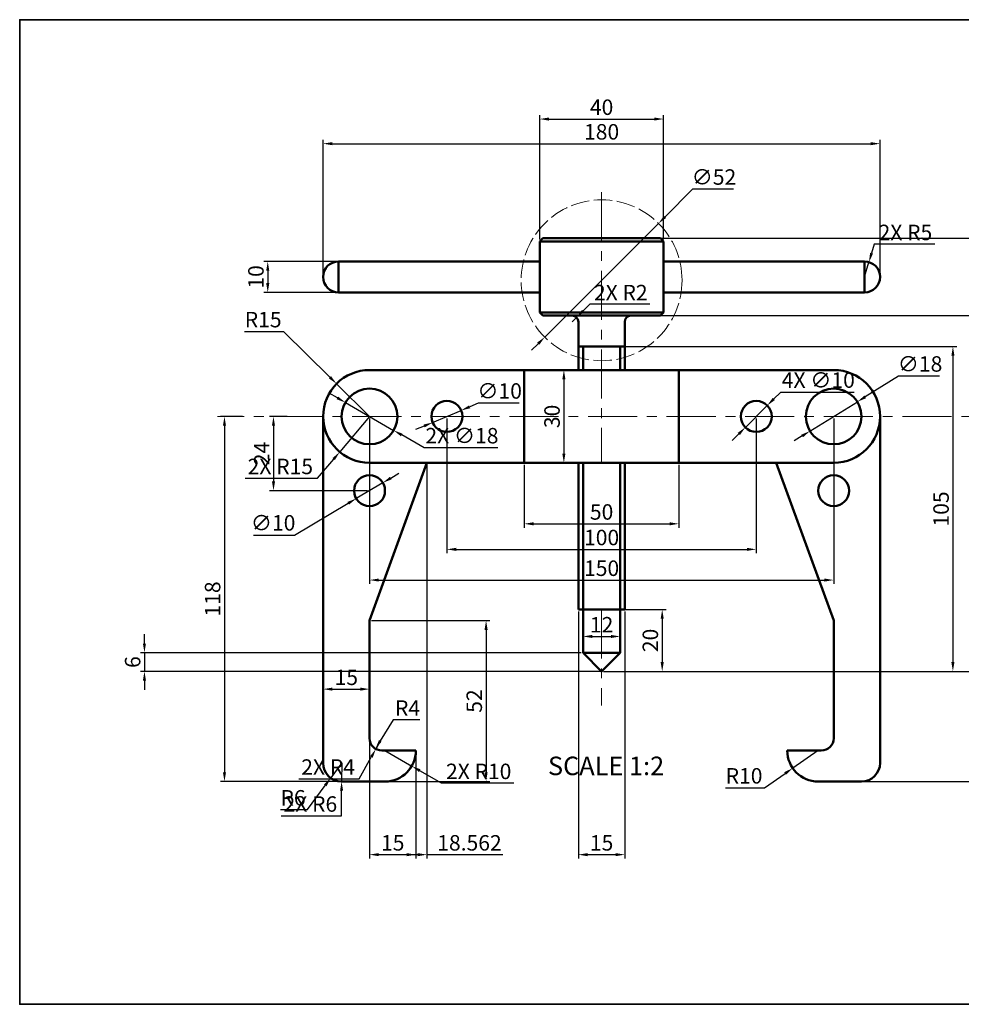
# Model space of a CAD drawing. Units: millimetres. Extents: x 535 to 1031, y 167 to 485.
# Tile 1 of 2: x 535 to 839, y 167 to 485. Entities that reach past the tile are written whole.
import ezdxf

# ---------------------------------------------------------------- set-up
doc = ezdxf.new("R2010")
doc.units = ezdxf.units.MM
doc.header["$LTSCALE"] = 0.5
doc.linetypes.add('ACAD_ISO02W100', pattern=[15, 12, -3])
doc.linetypes.add('CENTER', pattern=[50.8, 31.75, -6.35, 6.35, -6.35])
for name, color, linetype, lineweight in [('M-CNTR', 1, 'CENTER', 18), ('M-CONS', 8, 'ACAD_ISO02W100', 18), ('M-DIMS', 2, 'Continuous', 25), ('M-OUTL', 7, 'Continuous', 50), ('M-TEXT', 7, 'Continuous', 25), ('M-TTLB', 7, 'Continuous', 35)]:
    doc.layers.add(name, color=color, linetype=linetype, lineweight=lineweight)
doc.styles.get("Standard").update_dxf_attribs({"font": 'arial.ttf'})
doc.dimstyles.new('ISO-25', dxfattribs={"dimtxt": 5, "dimasz": 3, "dimexe": 1.25, "dimexo": 0.625, "dimtad": 1, "dimtoh": 1, "dimdec": 1, "dimtxsty": 'Standard', "dimcen": 2.5, "dimadec": 0, "dimazin": 0, "dimtfac": 1, "dimtdec": 1, "dimtmove": 0, "dimatfit": 3, "dimfxl": 1, "dimarcsym": 0})

# ---------------------------------------------------------------- blocks, each defined once
blk = doc.blocks.new('*D1')
at = {"layer": 'Defpoints', "color": 0, "transparency": 16777216}
for p in [(622.01, 356.84), (616.92, 332.84), (647.96, 332.84)]:
    blk.add_point(p, dxfattribs=at)
at = {"layer": 'M-DIMS', "color": 0, "lineweight": -2, "transparency": 16777216}
for p, q in [((621.39, 356.84), (615.67, 356.84)), ((616.92, 353.84), (616.92, 335.84)), ((647.33, 332.84), (615.67, 332.84))]:
    blk.add_line(p, q, dxfattribs=at)
at = {"layer": 'M-DIMS', "color": 0, "transparency": 16777216}
for points in [[(616.42, 353.84), (617.42, 353.84), (616.92, 356.84)], [(616.42, 335.84), (617.42, 335.84), (616.92, 332.84)]]:
    blk.add_solid(points, dxfattribs=at)
at = {"layer": 'M-DIMS', "color": 0, "transparency": 16777216, "insert": (613.78, 344.84), "char_height": 5, "attachment_point": 5, "rotation": 90}
blk.add_mtext('24', dxfattribs=at)
blk = doc.blocks.new('*D2')
at = {"layer": 'Defpoints', "color": 0, "transparency": 16777216}
for p in [(607.52, 356.84), (601.08, 238.84), (645.96, 238.84)]:
    blk.add_point(p, dxfattribs=at)
at = {"layer": 'M-DIMS', "color": 0, "lineweight": -2, "transparency": 16777216}
for p, q in [((606.9, 356.84), (599.83, 356.84)), ((601.08, 353.84), (601.08, 241.84)), ((645.33, 238.84), (599.83, 238.84))]:
    blk.add_line(p, q, dxfattribs=at)
at = {"layer": 'M-DIMS', "color": 0, "transparency": 16777216}
for points in [[(600.58, 353.84), (601.58, 353.84), (601.08, 356.84)], [(600.58, 241.84), (601.58, 241.84), (601.08, 238.84)]]:
    blk.add_solid(points, dxfattribs=at)
at = {"layer": 'M-DIMS', "color": 0, "transparency": 16777216, "insert": (597.9, 297.84), "char_height": 5, "attachment_point": 5, "rotation": 90}
blk.add_mtext('118', dxfattribs=at)
blk = doc.blocks.new('*D3')
at = {"layer": 'Defpoints', "color": 0, "transparency": 16777216}
for p in [(647.96, 290.84), (647.96, 238.84), (685.63, 238.84)]:
    blk.add_point(p, dxfattribs=at)
at = {"layer": 'M-DIMS', "color": 0, "lineweight": -2, "transparency": 16777216}
for p, q in [((648.58, 290.84), (686.88, 290.84)), ((685.63, 287.84), (685.63, 241.84)), ((648.58, 238.84), (686.88, 238.84))]:
    blk.add_line(p, q, dxfattribs=at)
at = {"layer": 'M-DIMS', "color": 0, "transparency": 16777216}
for points in [[(685.13, 287.84), (686.13, 287.84), (685.63, 290.84)], [(685.13, 241.84), (686.13, 241.84), (685.63, 238.84)]]:
    blk.add_solid(points, dxfattribs=at)
at = {"layer": 'M-DIMS', "color": 0, "transparency": 16777216, "insert": (682.45, 264.84), "char_height": 5, "attachment_point": 5, "rotation": 90}
blk.add_mtext('52', dxfattribs=at)
blk = doc.blocks.new('*D4')
at = {"layer": 'Defpoints', "color": 0, "transparency": 16777216}
for p in [(647.96, 268.69), (632.96, 265), (647.96, 265)]:
    blk.add_point(p, dxfattribs=at)
at = {"layer": 'M-DIMS', "color": 0, "lineweight": -2, "transparency": 16777216}
for p, q in [((632.96, 265.62), (632.96, 269.94)), ((635.96, 268.69), (644.96, 268.69)), ((647.96, 265.62), (647.96, 269.94))]:
    blk.add_line(p, q, dxfattribs=at)
at = {"layer": 'M-DIMS', "color": 0, "transparency": 16777216}
for points in [[(635.96, 269.19), (635.96, 268.19), (632.96, 268.69)], [(644.96, 269.19), (644.96, 268.19), (647.96, 268.69)]]:
    blk.add_solid(points, dxfattribs=at)
at = {"layer": 'M-DIMS', "color": 0, "transparency": 16777216, "insert": (640.46, 271.87), "char_height": 5, "attachment_point": 5}
blk.add_mtext('15', dxfattribs=at)
blk = doc.blocks.new('*D5')
at = {"layer": 'Defpoints', "color": 0, "transparency": 16777216}
for p in [(722.96, 294.43), (722.96, 274.43), (742.54, 274.43)]:
    blk.add_point(p, dxfattribs=at)
at = {"layer": 'M-DIMS', "color": 0, "lineweight": -2, "transparency": 16777216}
for p, q in [((723.58, 294.43), (743.79, 294.43)), ((742.54, 291.43), (742.54, 277.43)), ((723.58, 274.43), (743.79, 274.43))]:
    blk.add_line(p, q, dxfattribs=at)
at = {"layer": 'M-DIMS', "color": 0, "transparency": 16777216}
for points in [[(742.04, 291.43), (743.04, 291.43), (742.54, 294.43)], [(742.04, 277.43), (743.04, 277.43), (742.54, 274.43)]]:
    blk.add_solid(points, dxfattribs=at)
at = {"layer": 'M-DIMS', "color": 0, "transparency": 16777216, "insert": (739.36, 284.43), "char_height": 5, "attachment_point": 5, "rotation": 90}
blk.add_mtext('20', dxfattribs=at)
blk = doc.blocks.new('*D6')
at = {"layer": 'Defpoints', "color": 0, "transparency": 16777216}
for p in [(716.96, 288.28), (728.96, 288.28), (728.96, 285.72)]:
    blk.add_point(p, dxfattribs=at)
at = {"layer": 'M-DIMS', "color": 0, "lineweight": -2, "transparency": 16777216}
for p, q in [((716.96, 287.65), (716.96, 284.47)), ((728.96, 287.65), (728.96, 284.47)), ((719.96, 285.72), (725.96, 285.72))]:
    blk.add_line(p, q, dxfattribs=at)
at = {"layer": 'M-DIMS', "color": 0, "transparency": 16777216}
for points in [[(719.96, 286.22), (719.96, 285.22), (716.96, 285.72)], [(725.96, 286.22), (725.96, 285.22), (728.96, 285.72)]]:
    blk.add_solid(points, dxfattribs=at)
at = {"layer": 'M-DIMS', "color": 0, "transparency": 16777216, "insert": (722.96, 288.86), "char_height": 5, "attachment_point": 5}
blk.add_mtext('12', dxfattribs=at)
blk = doc.blocks.new('*D7')
at = {"layer": 'Defpoints', "color": 0, "transparency": 16777216}
for p in [(647.96, 356.84), (797.96, 356.84), (797.96, 303.95)]:
    blk.add_point(p, dxfattribs=at)
at = {"layer": 'M-DIMS', "color": 0, "lineweight": -2, "transparency": 16777216}
for p, q in [((647.96, 356.21), (647.96, 302.7)), ((797.96, 356.21), (797.96, 302.7)), ((650.96, 303.95), (794.96, 303.95))]:
    blk.add_line(p, q, dxfattribs=at)
at = {"layer": 'M-DIMS', "color": 0, "transparency": 16777216}
for points in [[(650.96, 304.45), (650.96, 303.45), (647.96, 303.95)], [(794.96, 304.45), (794.96, 303.45), (797.96, 303.95)]]:
    blk.add_solid(points, dxfattribs=at)
at = {"layer": 'M-DIMS', "color": 0, "transparency": 16777216, "insert": (722.96, 307.13), "char_height": 5, "attachment_point": 5}
blk.add_mtext('150', dxfattribs=at)
blk = doc.blocks.new('*D8')
at = {"layer": 'Defpoints', "color": 0, "transparency": 16777216}
for p in [(672.96, 356.84), (772.96, 356.84), (772.96, 313.87)]:
    blk.add_point(p, dxfattribs=at)
at = {"layer": 'M-DIMS', "color": 0, "lineweight": -2, "transparency": 16777216}
for p, q in [((672.96, 356.21), (672.96, 312.62)), ((772.96, 356.21), (772.96, 312.62)), ((675.96, 313.87), (769.96, 313.87))]:
    blk.add_line(p, q, dxfattribs=at)
at = {"layer": 'M-DIMS', "color": 0, "transparency": 16777216}
for points in [[(675.96, 314.37), (675.96, 313.37), (672.96, 313.87)], [(769.96, 314.37), (769.96, 313.37), (772.96, 313.87)]]:
    blk.add_solid(points, dxfattribs=at)
at = {"layer": 'M-DIMS', "color": 0, "transparency": 16777216, "insert": (722.96, 317.05), "char_height": 5, "attachment_point": 5}
blk.add_mtext('100', dxfattribs=at)
blk = doc.blocks.new('*D9')
at = {"layer": 'Defpoints', "color": 0, "transparency": 16777216}
for p in [(697.96, 341.84), (747.96, 341.84), (747.96, 322.13)]:
    blk.add_point(p, dxfattribs=at)
at = {"layer": 'M-DIMS', "color": 0, "lineweight": -2, "transparency": 16777216}
for p, q in [((697.96, 341.21), (697.96, 320.88)), ((747.96, 341.21), (747.96, 320.88)), ((700.96, 322.13), (744.96, 322.13))]:
    blk.add_line(p, q, dxfattribs=at)
at = {"layer": 'M-DIMS', "color": 0, "transparency": 16777216}
for points in [[(700.96, 322.63), (700.96, 321.63), (697.96, 322.13)], [(744.96, 322.63), (744.96, 321.63), (747.96, 322.13)]]:
    blk.add_solid(points, dxfattribs=at)
at = {"layer": 'M-DIMS', "color": 0, "transparency": 16777216, "insert": (722.96, 325.31), "char_height": 5, "attachment_point": 5}
blk.add_mtext('50', dxfattribs=at)
blk = doc.blocks.new('*D10')
at = {"layer": 'Defpoints', "color": 0, "transparency": 16777216}
for p in [(812.96, 445), (632.96, 401.93), (812.96, 401.93)]:
    blk.add_point(p, dxfattribs=at)
at = {"layer": 'M-DIMS', "color": 0, "lineweight": -2, "transparency": 16777216}
for p, q in [((632.96, 402.55), (632.96, 446.25)), ((812.96, 402.55), (812.96, 446.25)), ((635.96, 445), (809.96, 445))]:
    blk.add_line(p, q, dxfattribs=at)
at = {"layer": 'M-DIMS', "color": 0, "transparency": 16777216}
for points in [[(635.96, 445.5), (635.96, 444.5), (632.96, 445)], [(809.96, 445.5), (809.96, 444.5), (812.96, 445)]]:
    blk.add_solid(points, dxfattribs=at)
at = {"layer": 'M-DIMS', "color": 0, "transparency": 16777216, "insert": (722.96, 448.18), "char_height": 5, "attachment_point": 5}
blk.add_mtext('180', dxfattribs=at)
blk = doc.blocks.new('*D11')
at = {"layer": 'Defpoints', "color": 0, "transparency": 16777216}
for p in [(637.96, 406.93), (615.07, 396.93), (637.96, 396.93)]:
    blk.add_point(p, dxfattribs=at)
at = {"layer": 'M-DIMS', "color": 0, "lineweight": -2, "transparency": 16777216}
for p, q in [((637.33, 406.93), (613.82, 406.93)), ((615.07, 403.93), (615.07, 399.93)), ((637.33, 396.93), (613.82, 396.93))]:
    blk.add_line(p, q, dxfattribs=at)
at = {"layer": 'M-DIMS', "color": 0, "transparency": 16777216}
for points in [[(614.57, 403.93), (615.57, 403.93), (615.07, 406.93)], [(614.57, 399.93), (615.57, 399.93), (615.07, 396.93)]]:
    blk.add_solid(points, dxfattribs=at)
at = {"layer": 'M-DIMS', "color": 0, "transparency": 16777216, "insert": (611.89, 401.93), "char_height": 5, "attachment_point": 5, "rotation": 90}
blk.add_mtext('10', dxfattribs=at)
blk = doc.blocks.new('*D12')
at = {"layer": 'Defpoints', "color": 0, "transparency": 16777216}
for p in [(722.96, 414.43), (722.96, 274.43), (866.43, 274.43)]:
    blk.add_point(p, dxfattribs=at)
at = {"layer": 'M-DIMS', "color": 0, "lineweight": -2, "transparency": 16777216}
for p, q in [((723.58, 414.43), (867.68, 414.43)), ((866.43, 411.43), (866.43, 277.43)), ((723.58, 274.43), (867.68, 274.43))]:
    blk.add_line(p, q, dxfattribs=at)
at = {"layer": 'M-DIMS', "color": 0, "transparency": 16777216}
for points in [[(865.93, 411.43), (866.93, 411.43), (866.43, 414.43)], [(865.93, 277.43), (866.93, 277.43), (866.43, 274.43)]]:
    blk.add_solid(points, dxfattribs=at)
at = {"layer": 'M-DIMS', "color": 0, "transparency": 16777216, "insert": (863.25, 344.43), "char_height": 5, "attachment_point": 5, "rotation": 90}
blk.add_mtext('140', dxfattribs=at)
blk = doc.blocks.new('*D13')
at = {"layer": 'Defpoints', "color": 0, "transparency": 16777216}
for p in [(722.96, 379.43), (760.59, 274.43), (836.49, 274.43)]:
    blk.add_point(p, dxfattribs=at)
at = {"layer": 'M-DIMS', "color": 0, "lineweight": -2, "transparency": 16777216}
for p, q in [((723.58, 379.43), (837.74, 379.43)), ((836.49, 376.43), (836.49, 277.43)), ((761.21, 274.43), (837.74, 274.43))]:
    blk.add_line(p, q, dxfattribs=at)
at = {"layer": 'M-DIMS', "color": 0, "transparency": 16777216}
for points in [[(835.99, 376.43), (836.99, 376.43), (836.49, 379.43)], [(835.99, 277.43), (836.99, 277.43), (836.49, 274.43)]]:
    blk.add_solid(points, dxfattribs=at)
at = {"layer": 'M-DIMS', "color": 0, "transparency": 16777216, "insert": (833.31, 326.93), "char_height": 5, "attachment_point": 5, "rotation": 90}
blk.add_mtext('105', dxfattribs=at)
blk = doc.blocks.new('*D14')
at = {"layer": 'Defpoints', "color": 0, "transparency": 16777216}
for p in [(722.96, 389.43), (775.05, 274.43), (850.09, 274.43)]:
    blk.add_point(p, dxfattribs=at)
at = {"layer": 'M-DIMS', "color": 0, "lineweight": -2, "transparency": 16777216}
for p, q in [((723.58, 389.43), (851.34, 389.43)), ((850.09, 386.43), (850.09, 277.43)), ((775.67, 274.43), (851.34, 274.43))]:
    blk.add_line(p, q, dxfattribs=at)
at = {"layer": 'M-DIMS', "color": 0, "transparency": 16777216}
for points in [[(849.59, 386.43), (850.59, 386.43), (850.09, 389.43)], [(849.59, 277.43), (850.59, 277.43), (850.09, 274.43)]]:
    blk.add_solid(points, dxfattribs=at)
at = {"layer": 'M-DIMS', "color": 0, "transparency": 16777216, "insert": (846.91, 331.93), "char_height": 5, "attachment_point": 5, "rotation": 90}
blk.add_mtext('115', dxfattribs=at)
blk = doc.blocks.new('*D15')
at = {"layer": 'Defpoints', "color": 0, "transparency": 16777216}
for p in [(805.61, 361.57), (790.3, 352.1)]:
    blk.add_point(p, dxfattribs=at)
at = {"layer": 'M-DIMS', "color": 0, "lineweight": -2, "transparency": 16777216}
for p, q in [((818.95, 369.83), (808.16, 363.15)), ((832.19, 369.83), (818.95, 369.83)), ((790.3, 352.1), (805.61, 361.57)), ((787.75, 350.52), (785.2, 348.94))]:
    blk.add_line(p, q, dxfattribs=at)
at = {"layer": 'M-DIMS', "color": 0, "transparency": 16777216}
for points in [[(807.9, 363.58), (808.42, 362.73), (805.61, 361.57)], [(787.49, 350.94), (788.02, 350.09), (790.3, 352.1)]]:
    blk.add_solid(points, dxfattribs=at)
at = {"layer": 'M-DIMS', "color": 0, "transparency": 16777216, "insert": (825.88, 373.15), "char_height": 5, "attachment_point": 5}
blk.add_mtext('∅18', dxfattribs=at)
blk = doc.blocks.new('*D16')
at = {"layer": 'Defpoints', "color": 0, "transparency": 16777216}
for p in [(677.56, 358.78), (668.35, 354.89)]:
    blk.add_point(p, dxfattribs=at)
at = {"layer": 'M-DIMS', "color": 0, "lineweight": -2, "transparency": 16777216}
for p, q in [((683.09, 361.11), (680.33, 359.94)), ((696.3, 361.11), (683.09, 361.11)), ((668.35, 354.89), (677.56, 358.78)), ((665.58, 353.73), (662.82, 352.57))]:
    blk.add_line(p, q, dxfattribs=at)
at = {"layer": 'M-DIMS', "color": 0, "transparency": 16777216}
for points in [[(680.13, 360.4), (680.52, 359.48), (677.56, 358.78)], [(665.39, 354.19), (665.78, 353.27), (668.35, 354.89)]]:
    blk.add_solid(points, dxfattribs=at)
at = {"layer": 'M-DIMS', "color": 0, "transparency": 16777216, "insert": (690.01, 364.42), "char_height": 5, "attachment_point": 5}
blk.add_mtext('∅10', dxfattribs=at)
blk = doc.blocks.new('*D17')
at = {"layer": 'Defpoints', "color": 0, "transparency": 16777216}
for p in [(652.26, 335.39), (643.66, 330.29)]:
    blk.add_point(p, dxfattribs=at)
at = {"layer": 'M-DIMS', "color": 0, "lineweight": -2, "transparency": 16777216}
for p, q in [((654.84, 336.92), (657.42, 338.45)), ((652.26, 335.39), (643.66, 330.29)), ((623.72, 318.47), (641.07, 328.76)), ((610.51, 318.47), (623.72, 318.47))]:
    blk.add_line(p, q, dxfattribs=at)
at = {"layer": 'M-DIMS', "color": 0, "transparency": 16777216}
for points in [[(654.58, 337.35), (655.09, 336.49), (652.26, 335.39)], [(640.82, 329.19), (641.33, 328.33), (643.66, 330.29)]]:
    blk.add_solid(points, dxfattribs=at)
at = {"layer": 'M-DIMS', "color": 0, "transparency": 16777216, "insert": (616.81, 321.79), "char_height": 5, "attachment_point": 5}
blk.add_mtext('∅10', dxfattribs=at)
blk = doc.blocks.new('*D18')
at = {"layer": 'Defpoints', "color": 0, "transparency": 16777216}
for p in [(637.3, 367.39), (647.96, 356.84)]:
    blk.add_point(p, dxfattribs=at)
at = {"layer": 'M-DIMS', "color": 0, "lineweight": -2, "transparency": 16777216}
for p, q in [((607.6, 384.31), (620.21, 384.31)), ((620.21, 384.31), (635.17, 369.5)), ((647.96, 356.84), (637.3, 367.39))]:
    blk.add_line(p, q, dxfattribs=at)
at = {"layer": 'M-DIMS', "color": 0, "transparency": 16777216}
blk.add_solid([(635.52, 369.86), (634.81, 369.15), (637.3, 367.39)], dxfattribs=at)
at = {"layer": 'M-DIMS', "color": 0, "transparency": 16777216, "insert": (613.59, 387.49), "char_height": 5, "attachment_point": 5}
blk.add_mtext('R15', dxfattribs=at)
blk = doc.blocks.new('*D19')
at = {"layer": 'Defpoints', "color": 0, "transparency": 16777216}
for p in [(638.96, 244.84), (635.41, 240)]:
    blk.add_point(p, dxfattribs=at)
at = {"layer": 'M-DIMS', "color": 0, "lineweight": -2, "transparency": 16777216}
for p, q in [((638.96, 244.84), (635.41, 240)), ((627.89, 229.74), (633.63, 237.58)), ((619.2, 229.74), (627.89, 229.74))]:
    blk.add_line(p, q, dxfattribs=at)
at = {"layer": 'M-DIMS', "color": 0, "transparency": 16777216}
blk.add_solid([(633.23, 237.87), (634.04, 237.28), (635.41, 240)], dxfattribs=at)
at = {"layer": 'M-DIMS', "color": 0, "transparency": 16777216, "insert": (623.23, 232.92), "char_height": 5, "attachment_point": 5}
blk.add_mtext('R6', dxfattribs=at)
blk = doc.blocks.new('*D20')
at = {"layer": 'Defpoints', "color": 0, "transparency": 16777216}
for p in [(651.96, 252.84), (649.87, 249.42)]:
    blk.add_point(p, dxfattribs=at)
at = {"layer": 'M-DIMS', "color": 0, "lineweight": -2, "transparency": 16777216}
for p, q in [((655.61, 258.81), (651.43, 251.98)), ((664.27, 258.81), (655.61, 258.81))]:
    blk.add_line(p, q, dxfattribs=at)
at = {"layer": 'M-DIMS', "color": 0, "transparency": 16777216}
blk.add_solid([(651.01, 252.24), (651.86, 251.72), (649.87, 249.42)], dxfattribs=at)
at = {"layer": 'M-DIMS', "color": 0, "transparency": 16777216, "insert": (660.25, 261.93), "char_height": 5, "attachment_point": 5}
blk.add_mtext('R4', dxfattribs=at)
blk = doc.blocks.new('*D21')
at = {"layer": 'Defpoints', "color": 0, "transparency": 16777216}
for p in [(792.96, 248.84), (784.73, 243.15)]:
    blk.add_point(p, dxfattribs=at)
at = {"layer": 'M-DIMS', "color": 0, "lineweight": -2, "transparency": 16777216}
for p, q in [((792.96, 248.84), (784.73, 243.15)), ((775.59, 236.84), (782.26, 241.45)), ((763.04, 236.84), (775.59, 236.84))]:
    blk.add_line(p, q, dxfattribs=at)
at = {"layer": 'M-DIMS', "color": 0, "transparency": 16777216}
blk.add_solid([(781.98, 241.86), (782.54, 241.04), (784.73, 243.15)], dxfattribs=at)
at = {"layer": 'M-DIMS', "color": 0, "transparency": 16777216, "insert": (769, 240.02), "char_height": 5, "attachment_point": 5}
blk.add_mtext('R10', dxfattribs=at)
blk = doc.blocks.new('*D22')
at = {"layer": 'Defpoints', "color": 0, "transparency": 16777216}
for p in [(710.77, 371.84), (710.77, 341.84), (710.77, 341.84)]:
    blk.add_point(p, dxfattribs=at)
at = {"layer": 'M-DIMS', "color": 0, "lineweight": -2, "transparency": 16777216}
for p, q in [((711.4, 371.84), (712.02, 371.84)), ((710.77, 368.84), (710.77, 344.84)), ((711.4, 341.84), (712.02, 341.84))]:
    blk.add_line(p, q, dxfattribs=at)
at = {"layer": 'M-DIMS', "color": 0, "transparency": 16777216}
for points in [[(710.27, 368.84), (711.27, 368.84), (710.77, 371.84)], [(710.27, 344.84), (711.27, 344.84), (710.77, 341.84)]]:
    blk.add_solid(points, dxfattribs=at)
at = {"layer": 'M-DIMS', "color": 0, "transparency": 16777216, "insert": (707.59, 356.84), "char_height": 5, "attachment_point": 5, "rotation": 90}
blk.add_mtext('30', dxfattribs=at)
blk = doc.blocks.new('PULLER-JAW')
for p, q in [((-15, 24), (-15, -88)), ((0, -42), (18.56, 9)), ((0, -42), (0, -80)), ((15, -84), (4, -84)), ((15, -84), (15, -84)), ((5, -94), (-9, -94))]:
    blk.add_line(p, q)
blk.add_circle((0, 0), 5)
for centre, radius, start, end in [((4, -80), 4, 180, 270), ((5, -84), 10, 270, 0), ((-9, -88), 6, 180, 270)]:
    blk.add_arc(centre, radius, start, end)
blk = doc.blocks.new('TOMMY-BAR-END')
for p, q in [((0, 5), (0, -5)), ((65, 5), (0, 5)), ((0, -5), (65, -5))]:
    blk.add_line(p, q)
blk.add_arc((0, 0), 5, 90, 270)
blk = doc.blocks.new('CROSSHEAD-HOLE-PAIR')
for centre, radius in [((0, 0), 9), ((25, 0), 5)]:
    blk.add_circle(centre, radius)
blk = doc.blocks.new('*D26')
at = {"layer": 'Defpoints', "color": 0, "ltscale": 0.5, "transparency": 16777216}
for p in [(741.96, 414.43), (885.09, 414.43), (806.96, 238.84)]:
    blk.add_point(p, dxfattribs=at)
at = {"layer": 'M-DIMS', "color": 0, "lineweight": -2, "ltscale": 0.5, "transparency": 16777216}
for p, q in [((742.58, 414.43), (886.34, 414.43)), ((885.09, 241.84), (885.09, 411.43)), ((807.58, 238.84), (886.34, 238.84))]:
    blk.add_line(p, q, dxfattribs=at)
at = {"layer": 'M-DIMS', "color": 0, "ltscale": 0.5, "transparency": 16777216}
for points in [[(884.59, 411.43), (885.59, 411.43), (885.09, 414.43)], [(884.59, 241.84), (885.59, 241.84), (885.09, 238.84)]]:
    blk.add_solid(points, dxfattribs=at)
at = {"layer": 'M-DIMS', "color": 0, "ltscale": 0.5, "transparency": 16777216, "insert": (881.91, 326.63), "char_height": 5, "attachment_point": 5, "rotation": 90}
blk.add_mtext('175.6', dxfattribs=at)
blk = doc.blocks.new('*D27')
at = {"layer": 'Defpoints', "color": 0, "ltscale": 0.5, "transparency": 16777216}
for p in [(742.96, 452.96), (702.96, 413.43), (742.96, 413.43)]:
    blk.add_point(p, dxfattribs=at)
at = {"layer": 'M-DIMS', "color": 0, "lineweight": -2, "ltscale": 0.5, "transparency": 16777216}
for p, q in [((702.96, 414.05), (702.96, 454.21)), ((705.96, 452.96), (739.96, 452.96)), ((742.96, 414.05), (742.96, 454.21))]:
    blk.add_line(p, q, dxfattribs=at)
at = {"layer": 'M-DIMS', "color": 0, "ltscale": 0.5, "transparency": 16777216}
for points in [[(705.96, 453.46), (705.96, 452.46), (702.96, 452.96)], [(739.96, 453.46), (739.96, 452.46), (742.96, 452.96)]]:
    blk.add_solid(points, dxfattribs=at)
at = {"layer": 'M-DIMS', "color": 0, "ltscale": 0.5, "transparency": 16777216, "insert": (722.96, 456.14), "char_height": 5, "attachment_point": 5}
blk.add_mtext('40', dxfattribs=at)
blk = doc.blocks.new('*D28')
at = {"layer": 'Defpoints', "color": 0, "ltscale": 0.5, "transparency": 16777216}
for p in [(715.46, 294.43), (730.46, 294.43), (730.46, 215.19)]:
    blk.add_point(p, dxfattribs=at)
at = {"layer": 'M-DIMS', "color": 0, "lineweight": -2, "ltscale": 0.5, "transparency": 16777216}
for p, q in [((715.46, 293.8), (715.46, 213.94)), ((730.46, 293.8), (730.46, 213.94)), ((718.46, 215.19), (727.46, 215.19))]:
    blk.add_line(p, q, dxfattribs=at)
at = {"layer": 'M-DIMS', "color": 0, "ltscale": 0.5, "transparency": 16777216}
for points in [[(718.46, 215.69), (718.46, 214.69), (715.46, 215.19)], [(727.46, 215.69), (727.46, 214.69), (730.46, 215.19)]]:
    blk.add_solid(points, dxfattribs=at)
at = {"layer": 'M-DIMS', "color": 0, "ltscale": 0.5, "transparency": 16777216, "insert": (722.96, 218.36), "char_height": 5, "attachment_point": 5}
blk.add_mtext('15', dxfattribs=at)
blk = doc.blocks.new('*D29')
at = {"layer": 'Defpoints', "color": 0, "ltscale": 0.5, "transparency": 16777216}
for p in [(647.96, 252.84), (662.96, 248.84), (662.96, 215.19)]:
    blk.add_point(p, dxfattribs=at)
at = {"layer": 'M-DIMS', "color": 0, "lineweight": -2, "ltscale": 0.5, "transparency": 16777216}
for p, q in [((647.96, 252.21), (647.96, 213.94)), ((662.96, 248.21), (662.96, 213.94)), ((650.96, 215.19), (659.96, 215.19))]:
    blk.add_line(p, q, dxfattribs=at)
at = {"layer": 'M-DIMS', "color": 0, "ltscale": 0.5, "transparency": 16777216}
for points in [[(650.96, 215.69), (650.96, 214.69), (647.96, 215.19)], [(659.96, 215.69), (659.96, 214.69), (662.96, 215.19)]]:
    blk.add_solid(points, dxfattribs=at)
at = {"layer": 'M-DIMS', "color": 0, "ltscale": 0.5, "transparency": 16777216, "insert": (655.46, 218.36), "char_height": 5, "attachment_point": 5}
blk.add_mtext('15', dxfattribs=at)
blk = doc.blocks.new('*D30')
at = {"layer": 'Defpoints', "color": 0, "ltscale": 0.5, "transparency": 16777216}
for p in [(666.52, 341.84), (647.96, 290.84), (666.52, 215.19)]:
    blk.add_point(p, dxfattribs=at)
at = {"layer": 'M-DIMS', "color": 0, "lineweight": -2, "ltscale": 0.5, "transparency": 16777216}
for p, q in [((666.52, 341.21), (666.52, 213.94)), ((647.96, 290.21), (647.96, 213.94)), ((650.96, 215.19), (663.52, 215.19)), ((666.52, 215.19), (691, 215.19))]:
    blk.add_line(p, q, dxfattribs=at)
at = {"layer": 'M-DIMS', "color": 0, "ltscale": 0.5, "transparency": 16777216}
for points in [[(650.96, 215.69), (650.96, 214.69), (647.96, 215.19)], [(663.52, 215.69), (663.52, 214.69), (666.52, 215.19)]]:
    blk.add_solid(points, dxfattribs=at)
at = {"layer": 'M-DIMS', "color": 0, "ltscale": 0.5, "transparency": 16777216, "insert": (680.26, 218.36), "char_height": 5, "attachment_point": 5}
blk.add_mtext('18.562', dxfattribs=at)
blk = doc.blocks.new('*D31')
at = {"layer": 'Defpoints', "color": 0, "ltscale": 0.5, "transparency": 16777216}
for p in [(716.96, 280.43), (575.22, 274.43), (722.96, 274.43)]:
    blk.add_point(p, dxfattribs=at)
at = {"layer": 'M-DIMS', "color": 0, "lineweight": -2, "ltscale": 0.5, "transparency": 16777216}
for p, q in [((575.22, 283.43), (575.22, 286.43)), ((716.33, 280.43), (573.97, 280.43)), ((575.22, 280.43), (575.22, 274.43)), ((722.33, 274.43), (573.97, 274.43)), ((575.22, 271.43), (575.22, 268.43))]:
    blk.add_line(p, q, dxfattribs=at)
at = {"layer": 'M-DIMS', "color": 0, "ltscale": 0.5, "transparency": 16777216}
for points in [[(574.72, 283.43), (575.72, 283.43), (575.22, 280.43)], [(574.72, 271.43), (575.72, 271.43), (575.22, 274.43)]]:
    blk.add_solid(points, dxfattribs=at)
at = {"layer": 'M-DIMS', "color": 0, "ltscale": 0.5, "transparency": 16777216, "insert": (572.05, 277.43), "char_height": 5, "attachment_point": 5, "rotation": 90}
blk.add_mtext('6', dxfattribs=at)
blk = doc.blocks.new('*D32')
at = {"layer": 'Defpoints', "color": 0, "ltscale": 0.5, "transparency": 16777216}
for p in [(638.96, 244.84), (638.94, 238.84)]:
    blk.add_point(p, dxfattribs=at)
at = {"layer": 'M-DIMS', "color": 0, "lineweight": -2, "ltscale": 0.5, "transparency": 16777216}
for p, q in [((638.96, 244.84), (638.94, 238.84)), ((638.91, 227.73), (638.93, 235.84)), ((619.4, 227.73), (638.91, 227.73))]:
    blk.add_line(p, q, dxfattribs=at)
at = {"layer": 'M-DIMS', "color": 0, "ltscale": 0.5, "transparency": 16777216}
blk.add_solid([(638.43, 235.84), (639.43, 235.83), (638.94, 238.84)], dxfattribs=at)
at = {"layer": 'M-DIMS', "color": 0, "ltscale": 0.5, "transparency": 16777216, "insert": (628.84, 230.91), "char_height": 5, "attachment_point": 5}
blk.add_mtext('2X R6', dxfattribs=at)
blk = doc.blocks.new('*D33')
at = {"layer": 'Defpoints', "color": 0, "ltscale": 0.5, "transparency": 16777216}
for p in [(647.96, 356.84), (638.31, 345.34)]:
    blk.add_point(p, dxfattribs=at)
at = {"layer": 'M-DIMS', "color": 0, "lineweight": -2, "ltscale": 0.5, "transparency": 16777216}
for p, q in [((647.96, 356.84), (638.31, 345.34)), ((631.18, 336.84), (636.39, 343.05)), ((607.74, 336.84), (631.18, 336.84))]:
    blk.add_line(p, q, dxfattribs=at)
at = {"layer": 'M-DIMS', "color": 0, "ltscale": 0.5, "transparency": 16777216}
blk.add_solid([(636, 343.37), (636.77, 342.73), (638.31, 345.34)], dxfattribs=at)
at = {"layer": 'M-DIMS', "color": 0, "ltscale": 0.5, "transparency": 16777216, "insert": (619.14, 340.02), "char_height": 5, "attachment_point": 5}
blk.add_mtext('2X R15', dxfattribs=at)
blk = doc.blocks.new('*D34')
at = {"layer": 'Defpoints', "color": 0, "ltscale": 0.5, "transparency": 16777216}
for p in [(652.96, 248.84), (661.61, 243.83)]:
    blk.add_point(p, dxfattribs=at)
at = {"layer": 'M-DIMS', "color": 0, "lineweight": -2, "ltscale": 0.5, "transparency": 16777216}
for p, q in [((652.96, 248.84), (661.61, 243.83)), ((671.23, 238.28), (664.21, 242.33)), ((694.62, 238.28), (671.23, 238.28))]:
    blk.add_line(p, q, dxfattribs=at)
at = {"layer": 'M-DIMS', "color": 0, "ltscale": 0.5, "transparency": 16777216}
blk.add_solid([(664.46, 242.77), (663.96, 241.9), (661.61, 243.83)], dxfattribs=at)
at = {"layer": 'M-DIMS', "color": 0, "ltscale": 0.5, "transparency": 16777216, "insert": (683.24, 241.46), "char_height": 5, "attachment_point": 5}
blk.add_mtext('2X R10', dxfattribs=at)
blk = doc.blocks.new('*D35')
at = {"layer": 'Defpoints', "color": 0, "ltscale": 0.5, "transparency": 16777216}
for p in [(651.96, 252.84), (650, 249.34)]:
    blk.add_point(p, dxfattribs=at)
at = {"layer": 'M-DIMS', "color": 0, "lineweight": -2, "ltscale": 0.5, "transparency": 16777216}
for p, q in [((651.96, 252.84), (650, 249.34)), ((644.62, 239.72), (648.54, 246.73)), ((625.12, 239.72), (644.62, 239.72))]:
    blk.add_line(p, q, dxfattribs=at)
at = {"layer": 'M-DIMS', "color": 0, "ltscale": 0.5, "transparency": 16777216}
blk.add_solid([(648.1, 246.97), (648.97, 246.48), (650, 249.34)], dxfattribs=at)
at = {"layer": 'M-DIMS', "color": 0, "ltscale": 0.5, "transparency": 16777216, "insert": (634.56, 242.86), "char_height": 5, "attachment_point": 5}
blk.add_mtext('2X R4', dxfattribs=at)
blk = doc.blocks.new('*D36')
at = {"layer": 'Defpoints', "color": 0, "ltscale": 0.5, "transparency": 16777216}
for p in [(640.16, 361.33), (655.75, 352.34)]:
    blk.add_point(p, dxfattribs=at)
at = {"layer": 'M-DIMS', "color": 0, "lineweight": -2, "ltscale": 0.5, "transparency": 16777216}
for p, q in [((637.56, 362.83), (634.96, 364.33)), ((640.16, 361.33), (655.75, 352.34)), ((665.61, 346.65), (658.35, 350.84)), ((689.41, 346.65), (665.61, 346.65))]:
    blk.add_line(p, q, dxfattribs=at)
at = {"layer": 'M-DIMS', "color": 0, "ltscale": 0.5, "transparency": 16777216}
for points in [[(637.81, 363.26), (637.31, 362.4), (640.16, 361.33)], [(658.6, 351.27), (658.1, 350.41), (655.75, 352.34)]]:
    blk.add_solid(points, dxfattribs=at)
at = {"layer": 'M-DIMS', "color": 0, "ltscale": 0.5, "transparency": 16777216, "insert": (677.83, 349.97), "char_height": 5, "attachment_point": 5}
blk.add_mtext('2X ∅18', dxfattribs=at)
blk = doc.blocks.new('*D37')
at = {"layer": 'Defpoints', "color": 0, "ltscale": 0.5, "transparency": 16777216}
for p in [(776.49, 360.37), (769.42, 353.3)]:
    blk.add_point(p, dxfattribs=at)
at = {"layer": 'M-DIMS', "color": 0, "lineweight": -2, "ltscale": 0.5, "transparency": 16777216}
for p, q in [((780.73, 364.61), (778.61, 362.49)), ((804.62, 364.61), (780.73, 364.61)), ((769.42, 353.3), (776.49, 360.37)), ((767.3, 351.18), (765.18, 349.06))]:
    blk.add_line(p, q, dxfattribs=at)
at = {"layer": 'M-DIMS', "color": 0, "ltscale": 0.5, "transparency": 16777216}
for points in [[(778.26, 362.85), (778.97, 362.14), (776.49, 360.37)], [(766.95, 351.53), (767.65, 350.82), (769.42, 353.3)]]:
    blk.add_solid(points, dxfattribs=at)
at = {"layer": 'M-DIMS', "color": 0, "ltscale": 0.5, "transparency": 16777216, "insert": (792.99, 367.93), "char_height": 5, "attachment_point": 5}
blk.add_mtext('4X ∅10', dxfattribs=at)
blk = doc.blocks.new('*D38')
at = {"layer": 'Defpoints', "color": 0, "ltscale": 0.5, "transparency": 16777216}
for p in [(741.34, 419.22), (704.57, 382.46)]:
    blk.add_point(p, dxfattribs=at)
at = {"layer": 'M-DIMS', "color": 0, "lineweight": -2, "ltscale": 0.5, "transparency": 16777216}
for p, q in [((752.37, 430.25), (743.46, 421.34)), ((765.55, 430.25), (752.37, 430.25)), ((704.57, 382.46), (741.34, 419.22)), ((702.45, 380.33), (700.33, 378.21))]:
    blk.add_line(p, q, dxfattribs=at)
at = {"layer": 'M-DIMS', "color": 0, "ltscale": 0.5, "transparency": 16777216}
for points in [[(743.11, 421.7), (743.82, 420.99), (741.34, 419.22)], [(702.09, 380.69), (702.8, 379.98), (704.57, 382.46)]]:
    blk.add_solid(points, dxfattribs=at)
at = {"layer": 'M-DIMS', "color": 0, "ltscale": 0.5, "transparency": 16777216, "insert": (759.27, 433.57), "char_height": 5, "attachment_point": 5}
blk.add_mtext('∅52', dxfattribs=at)
blk = doc.blocks.new('*D39')
at = {"layer": 'Defpoints', "color": 0, "ltscale": 0.5, "transparency": 16777216}
for p in [(809.36, 406.73), (807.96, 401.93)]:
    blk.add_point(p, dxfattribs=at)
at = {"layer": 'M-DIMS', "color": 0, "lineweight": -2, "ltscale": 0.5, "transparency": 16777216}
for p, q in [((811.06, 412.48), (810.21, 409.61)), ((830.61, 412.48), (811.06, 412.48)), ((807.96, 401.93), (809.36, 406.73))]:
    blk.add_line(p, q, dxfattribs=at)
at = {"layer": 'M-DIMS', "color": 0, "ltscale": 0.5, "transparency": 16777216}
blk.add_solid([(809.73, 409.75), (810.69, 409.46), (809.36, 406.73)], dxfattribs=at)
at = {"layer": 'M-DIMS', "color": 0, "ltscale": 0.5, "transparency": 16777216, "insert": (821.14, 415.66), "char_height": 5, "attachment_point": 5}
blk.add_mtext('2X R5', dxfattribs=at)
blk = doc.blocks.new('*D40')
at = {"layer": 'Defpoints', "color": 0, "ltscale": 0.5, "transparency": 16777216}
for p in [(714.87, 388.84), (713.46, 387.43)]:
    blk.add_point(p, dxfattribs=at)
at = {"layer": 'M-DIMS', "color": 0, "lineweight": -2, "ltscale": 0.5, "transparency": 16777216}
for p, q in [((719.12, 393.08), (717, 390.96)), ((738.59, 393.08), (719.12, 393.08)), ((713.46, 387.43), (714.87, 388.84))]:
    blk.add_line(p, q, dxfattribs=at)
at = {"layer": 'M-DIMS', "color": 0, "ltscale": 0.5, "transparency": 16777216}
blk.add_solid([(716.64, 391.31), (717.35, 390.61), (714.87, 388.84)], dxfattribs=at)
at = {"layer": 'M-DIMS', "color": 0, "ltscale": 0.5, "transparency": 16777216, "insert": (729.16, 396.22), "char_height": 5, "attachment_point": 5}
blk.add_mtext('2X R2', dxfattribs=at)

msp = doc.modelspace()

# ---------------------------------------------------------------- linework, layer by layer
at = {"layer": 'M-CNTR'}
for p, q in [((722.956, 429.3139), (722.956, 341.8356)), ((861.4429, 356.8356), (598.8743, 356.8356)), ((722.956, 294.4294), (722.956, 263.3859))]:
    msp.add_line(p, q, dxfattribs=at)
at = {"layer": 'M-CONS'}
msp.add_circle((722.956, 400.8386), 26, dxfattribs=at)
at = {"layer": 'M-DIMS'}
msp.add_line((722.956, 274.4294), (707.9717, 274.4294), dxfattribs=at)
at = {"layer": 'M-OUTL'}
for p, q in [((703.956, 414.4294), (702.956, 413.4294)), ((722.956, 414.4294), (703.956, 414.4294)), ((716.956, 414.4294), (728.956, 414.4294)), ((741.956, 414.4294), (728.956, 414.4294)), ((741.956, 414.4294), (742.956, 413.4294)), ((702.956, 413.4294), (702.956, 390.4294)), ((702.956, 413.4294), (742.956, 413.4294)), ((742.956, 390.4294), (742.956, 413.4294)), ((702.956, 390.4294), (703.956, 389.4294)), ((702.956, 390.4294), (742.956, 390.4294)), ((741.956, 389.4294), (703.956, 389.4294)), ((742.956, 390.4294), (741.956, 389.4294)), ((715.456, 387.4294), (715.456, 371.8356)), ((730.456, 387.4294), (730.456, 371.8356)), ((730.456, 379.4294), (715.456, 379.4294)), ((716.956, 379.4294), (716.956, 371.8356)), ((728.956, 379.4294), (728.956, 371.8356)), ((647.956, 371.8356), (797.956, 371.8356)), ((697.956, 371.8356), (697.956, 341.8356)), ((747.956, 371.8356), (747.956, 341.8356)), ((647.956, 341.8356), (797.956, 341.8356)), ((715.456, 341.8356), (715.456, 294.4294)), ((716.956, 341.8356), (716.956, 280.4294)), ((728.956, 341.8356), (728.956, 280.4294)), ((730.456, 341.8356), (730.456, 294.4294)), ((715.456, 294.4294), (730.456, 294.4294)), ((716.956, 280.4294), (728.956, 280.4294)), ((716.956, 280.4294), (722.956, 274.4294)), ((728.956, 280.4294), (722.956, 274.4294))]:
    msp.add_line(p, q, dxfattribs=at)
for centre, radius, start, end in [((713.456, 387.4294), 2, 0, 90), ((732.456, 387.4294), 2, 90, 180), ((647.956, 356.8356), 15, 90, 270), ((797.956, 356.8356), 15, 270, 90)]:
    msp.add_arc(centre, radius, start, end, dxfattribs=at)
at = {"layer": 'M-TTLB'}
msp.add_lwpolyline([(1030.6713, 166.8201), (534.905, 166.8201), (534.905, 485.0728), (1030.6713, 485.0728)], close=True, dxfattribs=at)

# ---------------------------------------------------------------- block references
at = {"layer": 'M-OUTL'}
for name, p in [('TOMMY-BAR-END', (637.956, 401.9294)), ('CROSSHEAD-HOLE-PAIR', (647.956, 356.8356)), ('PULLER-JAW', (647.956, 332.8356))]:
    msp.add_blockref(name, p, dxfattribs=at)
at = {"layer": 'M-OUTL', "rotation": 180}
for name, p in [('TOMMY-BAR-END', (807.956, 401.9294)), ('CROSSHEAD-HOLE-PAIR', (797.956, 356.8356))]:
    msp.add_blockref(name, p, dxfattribs=at)
at = {"layer": 'M-OUTL', "extrusion": (0, 0, -1), "zscale": -1}
msp.add_blockref('PULLER-JAW', (-797.956, 332.8356), dxfattribs=at)

# ---------------------------------------------------------------- texts
at = {"layer": 'M-TEXT', "insert": (705.6331, 246.8827), "char_height": 6, "attachment_point": 1}
msp.add_mtext_dynamic_manual_height_columns('SCALE 1:2', width=41.24765, gutter_width=12.5, heights=[0], dxfattribs=at)

# ---------------------------------------------------------------- dimensions: what is measured, and where the dimension line sits
at = {"layer": 'M-DIMS', "ltscale": 0.5}
for base, p1, p2, override, picture, middle in [((742.956, 452.9639), (702.956, 413.4294), (742.956, 413.4294), {"dimdec": 0, "dimlfac": 1, "dimrnd": 0, "dimzin": 0, "dimdsep": 46, "dimlunit": 2}, '*D27', (722.956, 456.1418)), ((666.51847, 215.18558), (647.95599, 290.83558), (666.51847, 341.83558), {"dimdec": 3, "dimlfac": 1, "dimrnd": 0, "dimzin": 0, "dimdsep": 46, "dimlunit": 2}, '*D30', (680.26113, 218.36344)), ((730.456, 215.1856), (715.456, 294.4294), (730.456, 294.4294), {"dimdec": 0, "dimlfac": 1, "dimrnd": 0, "dimzin": 0, "dimdsep": 46, "dimlunit": 2}, '*D28', (722.956, 218.3634)), ((662.956, 215.1856), (647.956, 252.8356), (662.956, 248.8356), {"dimdec": 0, "dimlfac": 1, "dimrnd": 0, "dimzin": 0, "dimdsep": 46, "dimlunit": 2}, '*D29', (655.456, 218.3634))]:
    dim = msp.add_linear_dim(base=base, p1=p1, p2=p2, dimstyle='ISO-25', override=override, dxfattribs=at)
    dim.commit()
    dim.dimension.update_dxf_attribs({"geometry": picture, "text_midpoint": middle})
at = {"layer": 'M-DIMS'}
for base, p1, p2, picture, middle in [((812.956, 444.9987), (632.956, 401.9294), (812.956, 401.9294), '*D10', (722.956, 448.1766)), ((797.956, 303.9481), (647.956, 356.8356), (797.956, 356.8356), '*D7', (722.956, 307.126)), ((772.956, 313.8714), (672.956, 356.8356), (772.956, 356.8356), '*D8', (722.956, 317.0493)), ((747.956, 322.1348), (697.956, 341.8356), (747.956, 341.8356), '*D9', (722.956, 325.3127)), ((728.956, 285.7235), (716.956, 288.2782), (728.956, 288.2782), '*D6', (722.956, 288.8588)), ((647.956, 268.6922), (632.956, 264.9966), (647.956, 264.9966), '*D4', (640.456, 271.8701))]:
    dim = msp.add_linear_dim(base=base, p1=p1, p2=p2, dimstyle='ISO-25', override={"dimclrd": 0, "dimclre": 0, "dimclrt": 0}, dxfattribs=at)
    dim.commit()
    dim.dimension.update_dxf_attribs({"geometry": picture, "text_midpoint": middle})
at = {"layer": 'M-DIMS', "ltscale": 0.5}
dim = msp.add_diameter_dim_2p(p1=(704.5699, 382.4552), p2=(741.3421, 419.2221), dimstyle='ISO-25', override={"dimdec": 0, "dimlfac": 1, "dimrnd": 0, "dimzin": 0, "dimdsep": 46, "dimlunit": 2}, dxfattribs=at)
dim.commit()
dim.dimension.update_dxf_attribs({"geometry": '*D38', "text_midpoint": (759.2743, 430.2522), "dimtype": 163})
for center, mpoint, picture, middle in [((807.956, 401.9294), (809.3648, 406.7268), '*D39', (821.1449, 415.6616)), ((713.456, 387.4294), (714.8719, 388.8419), '*D40', (729.1648, 396.2164)), ((647.956, 356.8356), (638.3141, 345.3449), '*D33', (619.1436, 340.0153)), ((651.956, 252.8356), (650.0027, 249.3449), '*D35', (634.5591, 242.8616)), ((652.956, 248.8356), (661.6148, 243.833), '*D34', (683.2356, 241.4552)), ((638.956, 244.8356), (638.94, 238.8356), '*D32', (628.8413, 230.9078))]:
    dim = msp.add_radius_dim(center=center, mpoint=mpoint, text='2X <>', dimstyle='ISO-25', override={"dimdec": 0, "dimlfac": 1, "dimrnd": 0, "dimzin": 0, "dimdsep": 46, "dimlunit": 2}, dxfattribs=at)
    dim.commit()
    dim.dimension.update_dxf_attribs({"geometry": picture, "text_midpoint": middle})
at = {"layer": 'M-DIMS'}
for base, p1, p2, picture, middle in [((866.425, 274.4294), (722.956, 414.4294), (722.956, 274.4294), '*D12', (863.2471, 344.4294)), ((615.0686, 396.9294), (637.956, 406.9294), (637.956, 396.9294), '*D11', (611.8908, 401.9294)), ((850.0927, 274.4294), (722.956, 389.4294), (775.0492, 274.4294), '*D14', (846.9148, 331.9294)), ((836.4874, 274.4294), (722.956, 379.4294), (760.5871, 274.4294), '*D13', (833.3095, 326.9294)), ((710.7745, 341.8356), (710.7745, 371.8356), (710.7745, 341.8356), '*D22', (707.5949, 356.8356)), ((601.0823, 238.8356), (607.5229, 356.8356), (645.956, 238.8356), '*D2', (597.9045, 297.8356)), ((616.9153, 332.8356), (622.0141, 356.8356), (647.956, 332.8356), '*D1', (613.7801, 344.8356)), ((742.5428, 274.4294), (722.956, 294.4294), (722.956, 274.4294), '*D5', (739.365, 284.4294)), ((685.6321, 238.8356), (647.956, 290.8356), (647.956, 238.8356), '*D3', (682.4542, 264.8356))]:
    dim = msp.add_linear_dim(base=base, p1=p1, p2=p2, angle=90, dimstyle='ISO-25', override={"dimclrd": 0, "dimclre": 0, "dimclrt": 0}, dxfattribs=at)
    dim.commit()
    dim.dimension.update_dxf_attribs({"geometry": picture, "text_midpoint": middle})
at = {"layer": 'M-DIMS', "ltscale": 0.5}
for base, p1, p2, override, picture, middle in [((885.0929, 414.4294), (806.956, 238.8356), (741.956, 414.4294), {"dimdec": 1, "dimlfac": 1, "dimrnd": 0, "dimzin": 0, "dimdsep": 46, "dimlunit": 2}, '*D26', (881.915, 326.6325)), ((575.2243, 274.4294), (716.956, 280.4294), (722.956, 274.4294), {"dimdec": 0, "dimlfac": 1, "dimrnd": 0, "dimzin": 0, "dimdsep": 46, "dimlunit": 2}, '*D31', (572.0465, 277.4294))]:
    dim = msp.add_linear_dim(base=base, p1=p1, p2=p2, angle=90, dimstyle='ISO-25', override=override, dxfattribs=at)
    dim.commit()
    dim.dimension.update_dxf_attribs({"geometry": picture, "text_midpoint": middle})
at = {"layer": 'M-DIMS'}
for center, mpoint, picture, middle in [((647.956, 356.8356), (637.2972, 367.3898), '*D18', (613.5922, 384.3095)), ((651.956, 252.8356), (649.8698, 249.4227), '*D20', (660.253, 258.8081)), ((638.956, 244.8356), (635.4073, 239.9975), '*D19', (623.232, 229.7447))]:
    dim = msp.add_radius_dim(center=center, mpoint=mpoint, dimstyle='ISO-25', override={"dimclrd": 0, "dimclre": 0, "dimclrt": 0}, dxfattribs=at)
    dim.commit()
    dim.dimension.update_dxf_attribs({"geometry": picture, "text_midpoint": middle, "dimtype": 164})
for p1, p2, picture, middle in [((790.3037, 352.0982), (805.6083, 361.5729), '*D15', (825.8812, 369.8325)), ((652.2568, 335.3857), (643.6552, 330.2855), '*D17', (616.8073, 318.4681))]:
    dim = msp.add_diameter_dim_2p(p1=p1, p2=p2, dimstyle='ISO-25', override={"dimclrd": 0, "dimclre": 0, "dimclrt": 0}, dxfattribs=at)
    dim.commit()
    dim.dimension.update_dxf_attribs({"geometry": picture, "text_midpoint": middle, "dimtype": 163})
at = {"layer": 'M-DIMS', "ltscale": 0.5}
for p1, p2, text, picture, middle in [((769.4207, 353.2998), (776.4913, 360.3713), '4X <>', '*D37', (792.9907, 364.6142)), ((640.1599, 361.3324), (655.7521, 352.3388), '2X <>', '*D36', (677.8271, 346.6502))]:
    dim = msp.add_diameter_dim_2p(p1=p1, p2=p2, text=text, dimstyle='ISO-25', override={"dimdec": 0, "dimlfac": 1, "dimrnd": 0, "dimzin": 0, "dimdsep": 46, "dimlunit": 2}, dxfattribs=at)
    dim.commit()
    dim.dimension.update_dxf_attribs({"geometry": picture, "text_midpoint": middle, "dimtype": 163})
at = {"layer": 'M-DIMS'}
dim = msp.add_diameter_dim_2p(p1=(668.348, 354.8948), p2=(677.564, 358.7763), dimstyle='ISO-25', override={"dimclrd": 0, "dimclre": 0, "dimclrt": 0}, dxfattribs=at)
dim.commit()
dim.dimension.update_dxf_attribs({"geometry": '*D16', "text_midpoint": (690.0112, 364.4229)})
dim = msp.add_radius_dim(center=(792.956, 248.8356), mpoint=(784.7284, 243.1516), dimstyle='ISO-25', override={"dimclrd": 0, "dimclre": 0, "dimclrt": 0}, dxfattribs=at)
dim.commit()
dim.dimension.update_dxf_attribs({"geometry": '*D21', "text_midpoint": (769.001, 240.017)})

doc.saveas('drawing.dxf')
